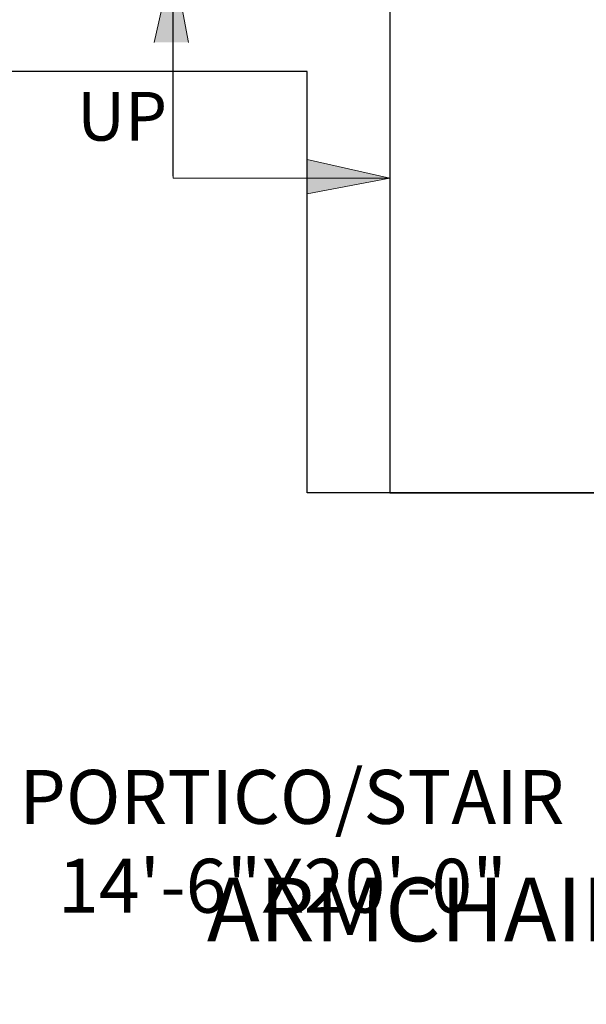
# Model space of a CAD drawing. Units: inches. Extents: x 0 to 4258, y 0 to 3769.
# Tile 15 of 30: x 3796 to 3859, y 3020 to 3128. Entities that reach past the tile are written whole.
import ezdxf

# ---------------------------------------------------------------- set-up
doc = ezdxf.new("R2010")
doc.units = ezdxf.units.IN
doc.header["$MEASUREMENT"] = 0
doc.layers.get('0').update_dxf_attribs({"color": 16})
for name, color, linetype, lineweight in [('A-ANNO-DIMS', 250, 'Continuous', 18), ('A-ANNO-SYMB', 250, 'Continuous', 18), ('A-ANNO-TEXT', 250, 'Continuous', 18), ('A-AREA-IDEN', 250, 'Continuous', 18), ('A-FLOR-STRS', 150, 'Continuous', 25)]:
    doc.layers.add(name, color=color, linetype=linetype, lineweight=lineweight)
doc.styles.get("Standard").update_dxf_attribs({"font": 'arial.ttf'})
doc.dimstyles.get("Standard").update_dxf_attribs({"dimtxt": 7, "dimasz": 0.18, "dimexe": 0.18, "dimexo": 0.0625, "dimgap": 0.09, "dimtad": 0, "dimtih": 1, "dimtoh": 1, "dimzin": 0, "dimdsep": 46, "dimlunit": 3, "dimtxsty": 'Standard', "dimcen": 0.09, "dimadec": 0, "dimazin": 0, "dimtfac": 1, "dimtofl": 0, "dimtmove": 0, "dimatfit": 3, "dimfxl": 1, "dimtolj": 1, "dimtzin": 0, "dimarcsym": 0})

# ---------------------------------------------------------------- blocks, each defined once
blk = doc.blocks.new('STAIR-DIRECTION-ARROW')
h = blk.add_hatch(color=256)
h.dxf.hatch_style = 1
h.paths.add_polyline_path([(14.74, 3.76), (14.74, 1.69), (23.85, 1.69)])
h.paths.add_polyline_path([(23.85, 1.69), (14.74, 1.69), (14.74, 0)])
for p, q in [((23.85, 1.69), (14.74, 3.76)), ((0, 1.69), (23.85, 1.69)), ((14.74, 0), (23.85, 1.69))]:
    blk.add_line(p, q)
blk = doc.blocks.new('*D52')
at = {"layer": 'A-ANNO-DIMS', "color": 0, "lineweight": -2, "transparency": 16777216}
for p, q in [((3889.6, 3030.12), (3889.42, 3030.12)), ((3889.6, 3026.46), (3889.6, 3030.3)), ((3914.27, 3030.12), (3889.78, 3030.12)), ((3914.45, 3026.46), (3914.45, 3030.3))]:
    blk.add_line(p, q, dxfattribs=at)
at = {"layer": 'A-ANNO-DIMS', "color": 0, "transparency": 16777216}
for points in [[(3889.78, 3030.15), (3889.78, 3030.09), (3889.6, 3030.12)], [(3914.27, 3030.15), (3914.27, 3030.09), (3914.45, 3030.12)]]:
    blk.add_solid(points, dxfattribs=at)
at = {"layer": 'Defpoints', "color": 0, "transparency": 16777216}
for p in [(3889.6, 3030.12), (3889.6, 3026.4), (3914.45, 3026.4)]:
    blk.add_point(p, dxfattribs=at)
at = {"layer": 'A-ANNO-DIMS', "color": 0, "transparency": 16777216, "insert": (3852.38, 3030.12), "char_height": 7, "attachment_point": 5}
blk.add_mtext('\\A1;ARMCHAIR 2\'-1"', dxfattribs=at)

msp = doc.modelspace()

# ---------------------------------------------------------------- hatches: boundary and pattern name
at = {"layer": 'A-ANNO-SYMB'}
h = msp.add_hatch(color=256, dxfattribs=at)
h.dxf.hatch_style = 1
h.paths.add_polyline_path([(3828.116, 3112.662), (3828.116, 3110.595), (3837.232, 3110.595)])
h.paths.add_polyline_path([(3837.232, 3110.595), (3828.116, 3110.595), (3828.116, 3108.903)])

# ---------------------------------------------------------------- linework, layer by layer
for p, q in [((3813.379, 3130.262), (3813.379, 3110.595)), ((3837.232, 3110.595), (3828.116, 3112.662)), ((3828.116, 3112.662), (3828.116, 3108.903)), ((3813.379, 3110.595), (3837.232, 3110.595)), ((3828.116, 3108.903), (3837.232, 3110.595))]:
    msp.add_line(p, q, dxfattribs=at)
at = {"layer": 'A-FLOR-STRS'}
for p, q in [((3837.232, 3130.262), (3837.232, 3075.983)), ((3828.116, 3122.34), (3786.102, 3122.34)), ((3828.116, 3075.983), (3828.116, 3122.34)), ((3861.804, 3075.983), (3828.116, 3075.983)), ((3837.232, 3075.983), (3861.804, 3075.983))]:
    msp.add_line(p, q, dxfattribs=at)

# ---------------------------------------------------------------- block references
at = {"layer": 'A-ANNO-SYMB', "rotation": 90.00000000000003}
msp.add_blockref('STAIR-DIRECTION-ARROW', (3815.049, 3110.82), dxfattribs=at)

# ---------------------------------------------------------------- texts
at = {"layer": 'A-ANNO-TEXT'}
msp.add_text('UP', height=5.3626, dxfattribs=at).set_placement((3802.81, 3114.747))
at = {"layer": 'A-AREA-IDEN'}
for s, p in [('PORTICO/STAIR', (3796.447, 3039.546)), ('14\'-6"X20\'-0"', (3800.699, 3029.764))]:
    msp.add_text(s, height=5.93898, dxfattribs=at).set_placement(p)

# ---------------------------------------------------------------- dimensions: what is measured, and where the dimension line sits
at = {"layer": 'A-ANNO-DIMS'}
dim = msp.add_linear_dim(base=(3889.595, 3030.125), p1=(3914.446, 3026.397), p2=(3889.595, 3026.397), angle=180, text='ARMCHAIR <>', dimstyle='Standard', override={"dimdec": 1, "dimlfac": 1, "dimrnd": 0, "dimzin": 1, "dimdsep": 46, "dimlunit": 4, "dimfrac": 2}, dxfattribs=at)
dim.commit()
dim.dimension.update_dxf_attribs({"geometry": '*D52', "text_midpoint": (3852.382, 3030.125)})

doc.saveas('drawing.dxf')
